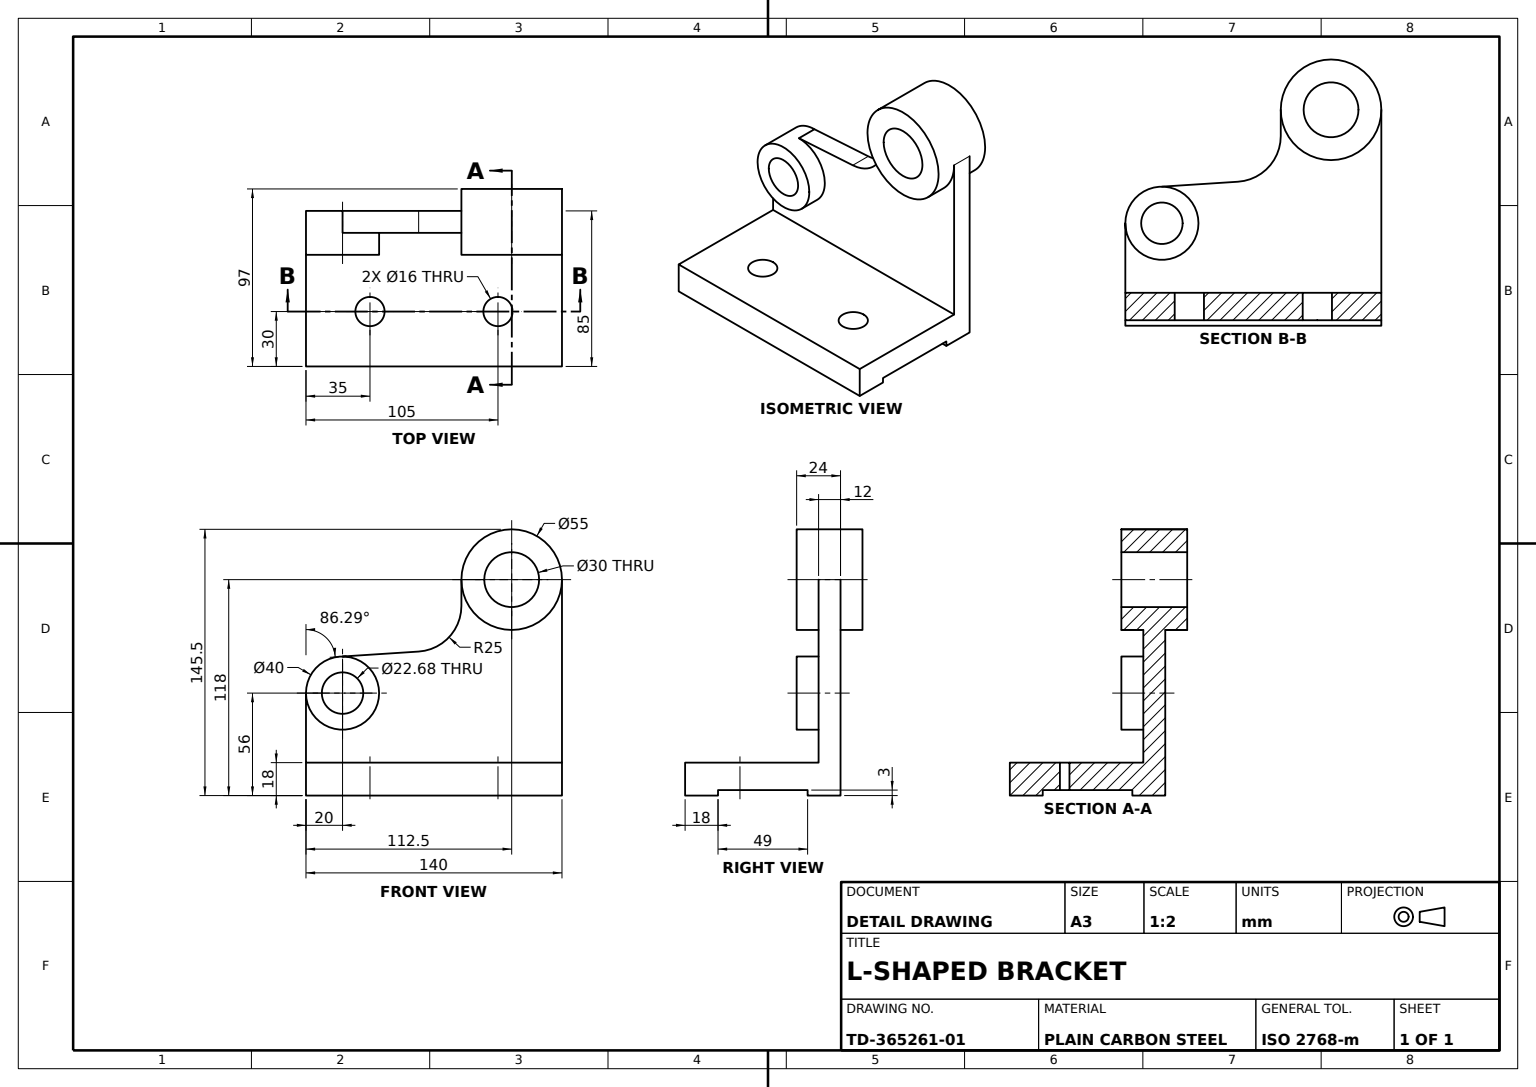
SolidWorks part; units mm, degrees
material "Plain Carbon Steel"
ref_plane "Front Plane" through (0, 0, 0) normal (0, 0, 1) x (1, 0, 0)
ref_plane "Top Plane" through (0, 0, 0) normal (0, 1, 0) x (1, 0, 0)
ref_plane "Right Plane" through (0, 0, 0) normal (1, 0, 0) x (0, 0, -1)
sketch "Base Plate Sketch" plane through (0, 0, 0) normal (0, 1, 0) x (1, 0, 0)
  line L0 (-70, 42.5) -> (70, 42.5)
  line L1 (70, 42.5) -> (70, -42.5)
  line L2 (70, -42.5) -> (-70, -42.5)
  line L3 (-70, -42.5) -> (-70, 42.5)
  line L4 (-70, 42.5) -> (70, -42.5) construction
  line L5 (70, 42.5) -> (-70, -42.5) construction
  point P2 (0, 0)
  dimension "D1" = 85
  dimension "D2" = 140
  dimension "D3" = 85
  dimension "D4" = 140
extrude "Base Plate 85x140x18" add sketch "Base Plate Sketch" along normal blind 18
sketch "Underside Groove Sketch" plane through (70, 0, 0) normal (1, 0, 0) x (0, 0, -1)
  line L0 (-42.5, 18) -> (-42.5, 0) construction
  line L1 (-42.5, 0) -> (42.5, 0) construction
  line L2 (-24.5, 0) -> (-24.5, 3)
  line L3 (-24.5, 3) -> (24.5, 3)
  line L4 (24.5, 3) -> (24.5, 0)
  line L5 (24.5, 0) -> (-24.5, 0)
  line L6 (42.5, 18) -> (42.5, 0) construction
  dimension "D1" = 18
  dimension "D2" = 18
  dimension "D3" = 3
extrude "Underside Groove" cut sketch "Underside Groove Sketch" against normal blind 140
sketch "Upright Wall Sketch" plane through (0, 18, 0) normal (0, 1, 0) x (1, 0, 0)
  line L0 (-70, 42.5) -> (-70, 30.5)
  line L1 (-70, 42.5) -> (-70, -42.5) construction
  line L2 (-70, 30.5) -> (70, 30.5)
  line L3 (70, -42.5) -> (70, 42.5) construction
  line L4 (70, 30.5) -> (70, 42.5)
  line L5 (70, 42.5) -> (-70, 42.5)
  dimension "D1" = 12
extrude "Upright Wall" add sketch "Upright Wall Sketch" along normal blind 100
sketch "Small Lug Ø40 Sketch" plane through (0, 0, -30.5) normal (0, 0, 1) x (1, 0, 0)
  line L0 (-70, 18) -> (70, 18) construction
  line L1 (-70, 118) -> (-70, 18) construction
  circle A0 centre (-50, 56) radius 20
  dimension "D1" = 40
  dimension "D2" = 38
extrude "Small Lug Ø40" add sketch "Small Lug Ø40 Sketch" along normal blind 12
sketch "Large Lug Ø55 Sketch" plane through (0, 0, -30.5) normal (0, 0, 1) x (1, 0, 0)
  line L0 (-70, 118) -> (70, 118) construction
  circle A0 centre (42.5, 118) radius 27.5
  dimension "D1" = 55
extrude "Large Lug Ø55" add sketch "Large Lug Ø55 Sketch" against normal blind 24
sketch "Large Lug Extension Sketch" plane through (0, 0, -30.5) normal (0, 0, 1) x (1, 0, 0)
  circle A0 centre (42.5, 118) radius 27.5
  dimension "D1" = 55
extrude "Large Lug Extension" add sketch "Large Lug Extension Sketch" along normal blind 12
sketch "Lug Relief Cut Sketch" plane through (0, 0, -30.5) normal (0, 0, 1) x (1, 0, 0)
  line L0 (15, 118) -> (15, 103.6431)
  line L2 (-50, 76) -> (-8.3842, 78.6954)
  line L3 (-70, 56) -> (-70, 118)
  line L4 (-70, 118) -> (15, 118)
  line L5 (-70, 118) -> (-70, 56) construction
  circle A0 centre (-50, 56) radius 20 construction
  arc A1 (15, 103.6431) -> (-8.3842, 78.6954) centre (-10, 103.6431) cw
  arc A2 (-50, 76) -> (-70, 56) centre (-50, 56) ccw
  circle A3 centre (42.5, 118) radius 27.5 construction
  dimension "D1" = 25
  dimension "D2" = 61.6158
extrude "Lug Relief Cut" cut sketch "Lug Relief Cut Sketch" against normal blind 12
sketch "Large Lug Bore Ø30 Sketch" plane through (0, 0, -18.5) normal (0, 0, 1) x (1, 0, 0)
  circle A0 centre (42.5, 118) radius 15
  dimension "D1" = 30
extrude "Large Lug Bore Ø30" cut sketch "Large Lug Bore Ø30 Sketch" against normal blind 36
sketch "Small Lug Bore Sketch" plane through (0, 0, -18.5) normal (0, 0, 1) x (1, 0, 0)
  circle A0 centre (-50, 56) radius 11.342
  dimension "D1" = 22.684
extrude "Small Lug Bore" cut sketch "Small Lug Bore Sketch" against normal blind 36
sketch "Base Mounting Hole 1 Ø16 Sketch" plane through (0, 18, 0) normal (0, 1, 0) x (1, 0, 0)
  line L0 (-70, -42.5) -> (70, -42.5) construction
  line L1 (-70, 30.5) -> (-70, -42.5) construction
  circle A0 centre (-35, -12.5) radius 8
  dimension "D3" = 16
  dimension "D1" = 30
  dimension "D2" = 35
extrude "Base Mounting Hole 1 Ø16" cut sketch "Base Mounting Hole 1 Ø16 Sketch" against normal blind 15
sketch "Base Mounting Hole 2 Ø16 Sketch" plane through (0, 18, 0) normal (0, 1, 0) x (1, 0, 0)
  line L0 (70, -42.5) -> (70, 30.5) construction
  line L1 (-70, -42.5) -> (70, -42.5) construction
  circle A0 centre (35, -12.5) radius 8
  dimension "D3" = 16
  dimension "D1" = 35
  dimension "D2" = 30
extrude "Base Mounting Hole 2 Ø16" cut sketch "Base Mounting Hole 2 Ø16 Sketch" against normal blind 15
